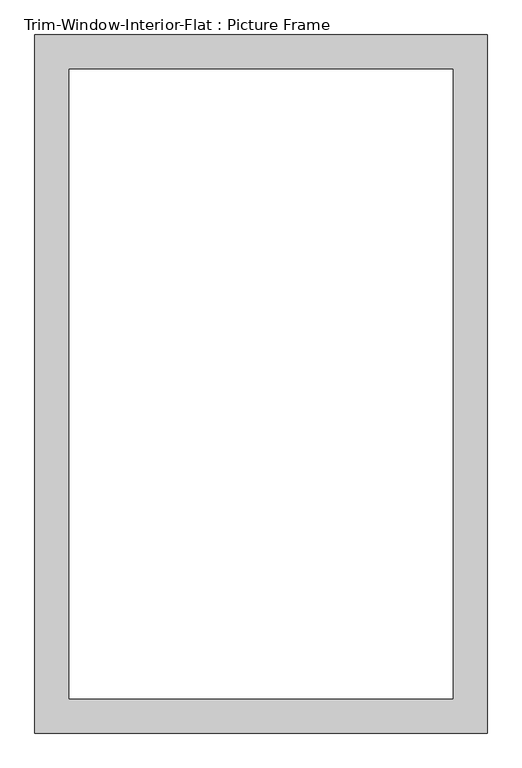
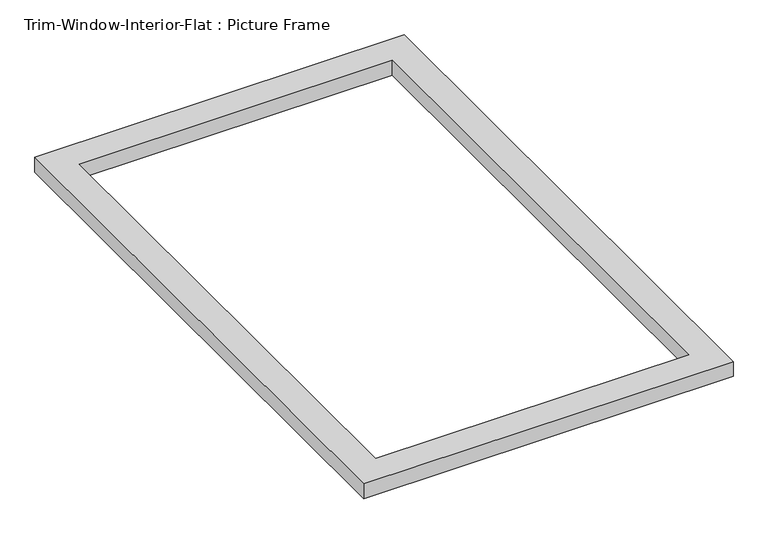
"""IFC4 building model written with IfcOpenShell, lengths in millimetres: proxy geometry, Trim-Window-Interior-Flat : Picture Frame."""

from ifc_helpers import new_model, si_unit, origin, origin_with_axes, place, context, project, spatial, polyline, outline, extrude, source, transform, mapped, element, save


def trim_window_interior_flat_picture_frame_d728ed12(model_context):
    return source(origin(), model_context, "Body", "SweptSolid", [
        extrude(outline(polyline([(374.65, 44.45), (374.65, -1111.25), (-374.65, -1111.25), (-374.65, 44.45), (374.65, 44.45)]), holes=[polyline([(317.5, -12.7), (-317.5, -12.7), (-317.5, -1054.1), (317.5, -1054.1), (317.5, -12.7)])]), origin_with_axes(), (0.0, 0.0, 1.0), 31.75),
    ])


if __name__ == "__main__":
    model = new_model("IFC4")
    model_context = context("Model", 3, world=origin())
    ifc_project = project(units=[si_unit("LENGTHUNIT", "METRE", prefix="MILLI")], contexts=[model_context])
    site = spatial("IfcSite", under=ifc_project)
    building = spatial("IfcBuilding", under=site)
    placement = place(None, origin())
    trim_window_interior_flat_picture_frame_shape = trim_window_interior_flat_picture_frame_d728ed12(model_context)
    element("IfcBuildingElementProxy", 1, Name="Trim-Window-Interior-Flat : Picture Frame", ObjectType="Trim-Window-Interior-Flat : Picture Frame", at=placement, inside=building, context=model_context, shape_type="MappedRepresentation", body=[
        mapped(trim_window_interior_flat_picture_frame_shape, transform((0.0, 0.0, 0.0), x_axis=(1.0, 0.0, 0.0), y_axis=(0.0, 1.0, 0.0), z_axis=(0.0, 0.0, 1.0))),
    ])
    save(model, "model.ifc")

# Revit data of these elements
# Type "Trim-Window-Interior-Flat : Picture Frame"
#   Trim Thickness_Picture Frame = 0' - 1 1/4"
#   Trim Width = 0' - 2 1/4"
#   Trim Thickness_with Sill = 0' - 0 3/4"
#   Sill Thickness = 0' - 1 1/4"
#   Opening Width [instance default] = 2' - 0"
#   Opening Height [instance default] = 3' - 0"
#   Default Elevation = 4' - 0"
#   Sill = no
#   Picture Frame = yes
#   Trim Material [instance default] = none
# Element 1 (IfcBuildingElementProxy, "Trim-Window-Interior-Flat : Picture Frame")
#   Opening Width = 2' - 2"
#   Opening Height = 3' - 6"
#   Trim Material = Wood - Stained
#   Materials on its faces: "Wood - Stained"
# Materials
#   "Wood - Stained": class "Wood", colour RGB 224 178 126, transparency 0, Cost = 0
